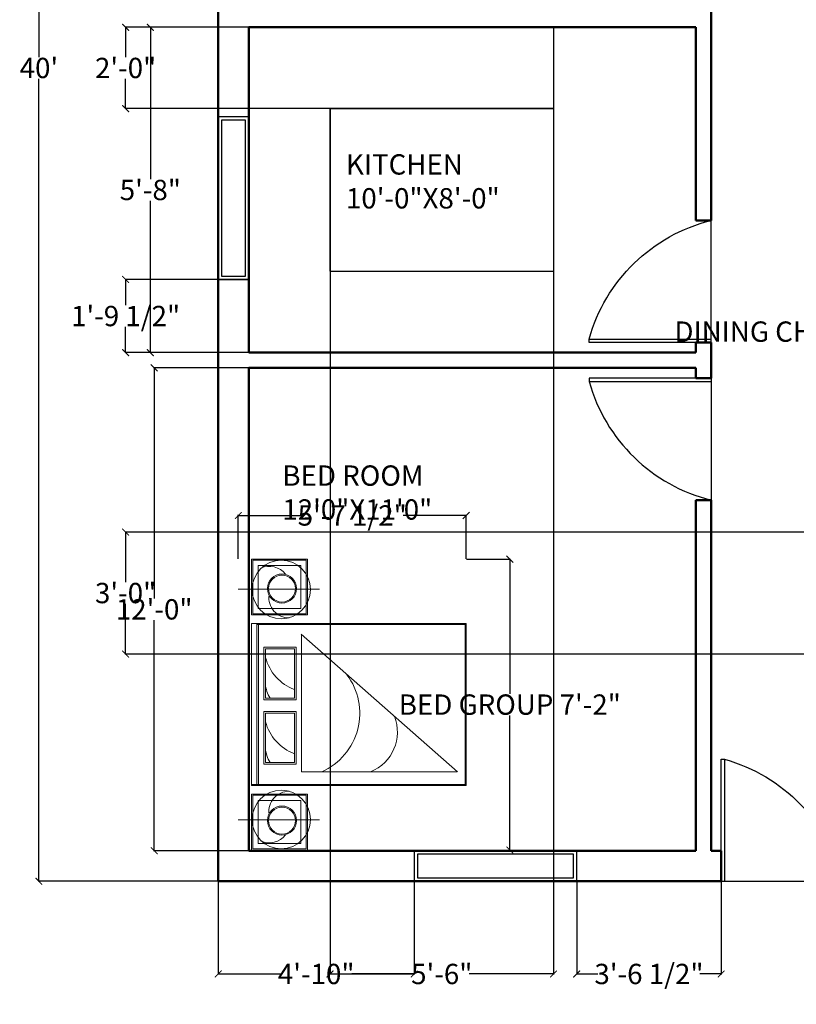
# Model space of a CAD drawing. Units: inches. Extents: x -40 to 418, y 1212 to 1787.
# Tile 1 of 3: x -40 to 189, y 1212 to 1503. Entities that reach past the tile are written whole.
import ezdxf

# ---------------------------------------------------------------- set-up
doc = ezdxf.new("R2010")
doc.units = ezdxf.units.IN
doc.header["$MEASUREMENT"] = 0
for name, color, linetype, lineweight in [('A-ANNO-DIMS', 2, 'Continuous', 18), ('A-AREA-IDEN', 7, 'Continuous', 25), ('A-DOOR', 4, 'Continuous', 25), ('A-FLOR-FIXT', 9, 'Continuous', 25), ('A-FURN', 8, 'Continuous', 18), ('A-GLAZ', 4, 'Continuous', 25), ('A-WALL', 7, 'Continuous', 50)]:
    doc.layers.add(name, color=color, linetype=linetype, lineweight=lineweight)
doc.styles.get("Standard").update_dxf_attribs({"font": 'arial.ttf'})
doc.dimstyles.get("Standard").update_dxf_attribs({"dimtxt": 6, "dimasz": 2, "dimexe": 0.18, "dimexo": 0.0625, "dimgap": 0.09, "dimtad": 0, "dimtih": 1, "dimtoh": 1, "dimdec": 0, "dimzin": 0, "dimdsep": 46, "dimlunit": 4, "dimtxsty": 'Standard', "dimblk": 'ARCHTICK', "dimcen": 0.09, "dimadec": 0, "dimazin": 0, "dimtfac": 1, "dimtdec": 0, "dimtofl": 0, "dimtmove": 0, "dimatfit": 3, "dimldrblk": 'ARCHTICK', "dimfxl": 1, "dimtolj": 1, "dimtzin": 0, "dimarcsym": 0})

# ---------------------------------------------------------------- blocks, each defined once
blk = doc.blocks.new('_ArchTick')
at = {"color": 0, "linetype": 'ByBlock', "const_width": 0.15}
blk.add_lwpolyline([(-0.5, -0.5), (0.5, 0.5)], dxfattribs=at)
blk = doc.blocks.new('*D5')
at = {"layer": 'A-ANNO-DIMS', "color": 0, "lineweight": -2, "transparency": 16777216}
for p, q in [((18.37, 1728.64), (-34.7, 1728.64)), ((-34.52, 1728.64), (-34.52, 1491.79)), ((-34.52, 1248.64), (-34.52, 1485.48)), ((18.37, 1248.64), (-34.7, 1248.64))]:
    blk.add_line(p, q, dxfattribs=at)
at = {"layer": 'Defpoints', "color": 0, "transparency": 16777216}
for p in [(-34.52, 1728.64), (18.43, 1728.64), (18.43, 1248.64)]:
    blk.add_point(p, dxfattribs=at)
at = {"layer": 'A-ANNO-DIMS', "color": 0, "lineweight": -2, "transparency": 16777216, "xscale": 2, "yscale": 2, "zscale": 2}
for p, rotation in [((-34.52, 1728.64), 90), ((-34.52, 1248.64), 270)]:
    blk.add_blockref('_ArchTick', p, dxfattribs=dict(at, rotation=rotation))
at = {"layer": 'A-ANNO-DIMS', "color": 0, "transparency": 16777216, "insert": (-34.52, 1488.64), "char_height": 6, "attachment_point": 5}
blk.add_mtext("\\A1;40'", dxfattribs=at)
blk = doc.blocks.new('*D8')
at = {"layer": 'A-ANNO-DIMS', "color": 0, "lineweight": -2, "transparency": 16777216}
for p, q in [((27.37, 1500.64), (-1.8, 1500.64)), ((-1.62, 1500.64), (-1.62, 1455.79)), ((-1.62, 1404.64), (-1.62, 1449.48)), ((27.37, 1404.64), (-1.8, 1404.64))]:
    blk.add_line(p, q, dxfattribs=at)
at = {"layer": 'Defpoints', "color": 0, "transparency": 16777216}
for p in [(-1.62, 1500.64), (27.43, 1500.64), (27.43, 1404.64)]:
    blk.add_point(p, dxfattribs=at)
at = {"layer": 'A-ANNO-DIMS', "color": 0, "lineweight": -2, "transparency": 16777216, "xscale": 2, "yscale": 2, "zscale": 2}
for p, rotation in [((-1.62, 1500.64), 90), ((-1.62, 1404.64), 270)]:
    blk.add_blockref('_ArchTick', p, dxfattribs=dict(at, rotation=rotation))
at = {"layer": 'A-ANNO-DIMS', "color": 0, "transparency": 16777216, "insert": (-1.62, 1452.64), "char_height": 6, "attachment_point": 5}
blk.add_mtext('\\A1;5\'-8"', dxfattribs=at)
blk = doc.blocks.new('*D9')
at = {"layer": 'A-ANNO-DIMS', "color": 0, "lineweight": -2, "transparency": 16777216}
for p, q in [((27.37, 1400.14), (-0.66, 1400.14)), ((-0.48, 1400.14), (-0.48, 1332.04)), ((-0.48, 1257.64), (-0.48, 1325.73)), ((27.37, 1257.64), (-0.66, 1257.64))]:
    blk.add_line(p, q, dxfattribs=at)
at = {"layer": 'Defpoints', "color": 0, "transparency": 16777216}
for p in [(-0.48, 1400.14), (27.43, 1400.14), (27.43, 1257.64)]:
    blk.add_point(p, dxfattribs=at)
at = {"layer": 'A-ANNO-DIMS', "color": 0, "lineweight": -2, "transparency": 16777216, "xscale": 2, "yscale": 2, "zscale": 2}
for p, rotation in [((-0.48, 1400.14), 90), ((-0.48, 1257.64), 270)]:
    blk.add_blockref('_ArchTick', p, dxfattribs=dict(at, rotation=rotation))
at = {"layer": 'A-ANNO-DIMS', "color": 0, "transparency": 16777216, "insert": (-0.48, 1328.89), "char_height": 6, "attachment_point": 5}
blk.add_mtext('\\A1;12\'-0"', dxfattribs=at)
blk = doc.blocks.new('DESDFGHJUI')
for p, q in [((-198.91, 1688.99), (-198.91, 1729.95)), ((-82.83, 1688.99), (-82.83, 1729.95)), ((-214.04, 1695.16), (-214.04, 1723.24)), ((-214.04, 1723.24), (-185.96, 1723.24)), ((-213.5, 1695.7), (-213.5, 1722.7)), ((-213.5, 1722.7), (-186.5, 1722.7)), ((-210.8, 1698.4), (-210.8, 1720)), ((-210.8, 1720), (-189.2, 1720)), ((-189.2, 1720), (-189.2, 1698.4)), ((-186.5, 1722.7), (-186.5, 1695.7)), ((-185.96, 1723.24), (-185.96, 1695.16)), ((-181.64, 1723.24), (-181.64, 1615.24)), ((-181.64, 1723.24), (-100.1, 1723.24)), ((-181.64, 1720.54), (-100.1, 1720.54)), ((-181.64, 1719.73), (-100.1, 1719.73)), ((-181.1, 1723.24), (-181.1, 1615.24)), ((-100.64, 1720.54), (-100.64, 1615.24)), ((-100.1, 1723.24), (-100.1, 1615.24)), ((-67.7, 1723.24), (-95.78, 1723.24)), ((-95.78, 1723.24), (-95.78, 1695.16)), ((-68.24, 1722.7), (-95.24, 1722.7)), ((-95.24, 1722.7), (-95.24, 1695.7)), ((-70.94, 1720), (-92.54, 1720)), ((-92.54, 1720), (-92.54, 1698.4)), ((-70.94, 1698.4), (-70.94, 1720)), ((-68.24, 1695.7), (-68.24, 1722.7)), ((-67.7, 1695.16), (-67.7, 1723.24)), ((-170.78, 1700.83), (-170.78, 1717.03)), ((-170.78, 1717.03), (-144.32, 1717.03)), ((-169.97, 1701.64), (-169.97, 1716.22)), ((-169.97, 1716.22), (-145.13, 1716.22)), ((-145.13, 1716.22), (-145.13, 1701.64)), ((-144.32, 1717.03), (-144.32, 1700.83)), ((-138.48, 1700.83), (-138.48, 1717.03)), ((-138.48, 1717.03), (-112.02, 1717.03)), ((-137.67, 1701.64), (-137.67, 1716.22)), ((-137.67, 1716.22), (-112.83, 1716.22)), ((-112.83, 1716.22), (-112.83, 1701.64)), ((-112.02, 1717.03), (-112.02, 1700.83)), ((-170.78, 1700.83), (-144.32, 1700.83)), ((-169.97, 1701.64), (-145.13, 1701.64)), ((-138.48, 1700.83), (-112.02, 1700.83)), ((-137.67, 1701.64), (-112.83, 1701.64)), ((-185.96, 1695.16), (-214.04, 1695.16)), ((-186.5, 1695.7), (-213.5, 1695.7)), ((-189.2, 1698.4), (-210.8, 1698.4)), ((-174.68, 1619.61), (-105.47, 1698.21)), ((-174.64, 1619.8), (-174.64, 1698.13)), ((-174.64, 1698.13), (-105.54, 1698.13)), ((-95.78, 1695.16), (-67.7, 1695.16)), ((-95.24, 1695.7), (-68.24, 1695.7)), ((-92.54, 1698.4), (-70.94, 1698.4)), ((-131.52, 1615.74), (-181.64, 1615.74)), ((-100.1, 1615.24), (-181.64, 1615.24)), ((-100.1, 1615.78), (-175.16, 1615.78))]:
    blk.add_line(p, q)
for centre, radius in [((-198.74, 1708.29), 14.73), ((-83.01, 1708.29), 14.73), ((-199.23, 1707.96), 7.32), ((-199.23, 1707.96), 6.78), ((-82.52, 1707.96), 7.32), ((-82.52, 1707.96), 6.78)]:
    blk.add_circle(centre, radius)
for centre, radius, start, end in [((-200.04, 1714.33), 10.36, 155.9567, 231.7564), ((-194.74, 1704.25), 10.3, 0.4104, 96.764), ((-161.57, 1700.2), 16.13, 94.4656, 121.4122), ((-143.54, 1693.44), 23.54, 104.6626, 159.6122), ((-129.26, 1700.2), 16.13, 94.4656, 121.4122), ((-111.24, 1693.44), 23.54, 104.6626, 159.6122), ((-87.01, 1704.25), 10.3, 83.236, 179.5896), ((-81.71, 1714.33), 10.36, 308.2436, 24.0433), ((-145.2, 1701.08), 32.28, 204.0563, 306.8492), ((-154.7, 1671.44), 21.57, 202.1275, 291.5505)]:
    blk.add_arc(centre, radius, start, end)
blk = doc.blocks.new('EREGTHYGUI')
for p, q in [((195.43, 1607.14), (194.43, 1607.14)), ((194.43, 1607.14), (194.43, 1571.14)), ((195.43, 1571.14), (195.43, 1607.14)), ((195.43, 1571.14), (159.43, 1571.14))]:
    blk.add_line(p, q)
blk.add_arc((207.79, 1559.14), 49.82, 105.5486, 166.0653)
blk = doc.blocks.new('WIN-48IN')
for points in [[(0, 0), (9, 0), (9, 48), (0, 48)], [(1, 1), (8, 1), (8, 47), (1, 47)]]:
    blk.add_lwpolyline(points, close=True)
blk = doc.blocks.new('*D21')
at = {"layer": 'A-ANNO-DIMS', "color": 0, "lineweight": -2, "transparency": 16777216}
for p, q in [((253.98, 1414.1), (253.98, 1410.66)), ((276.18, 1414.1), (276.18, 1410.66)), ((253.98, 1410.84), (251.98, 1410.84)), ((276.18, 1410.84), (253.98, 1410.84))]:
    blk.add_line(p, q, dxfattribs=at)
at = {"layer": 'Defpoints', "color": 0, "transparency": 16777216}
for p in [(253.98, 1414.17), (276.18, 1414.17), (253.98, 1410.84)]:
    blk.add_point(p, dxfattribs=at)
at = {"layer": 'A-ANNO-DIMS', "color": 0, "lineweight": -2, "transparency": 16777216, "xscale": 2, "yscale": 2, "zscale": 2}
for p, rotation in [((253.98, 1410.84), 179.9999999999912), ((276.18, 1410.84), 359.9999999999912)]:
    blk.add_blockref('_ArchTick', p, dxfattribs=dict(at, rotation=rotation))
at = {"layer": 'A-ANNO-DIMS', "color": 0, "transparency": 16777216, "insert": (201.38, 1410.84), "char_height": 6, "attachment_point": 5}
blk.add_mtext('\\A1;DINING CHAIR 1\'-10" TYP.', dxfattribs=at)
blk = doc.blocks.new('*D25')
at = {"layer": 'A-ANNO-DIMS', "color": 0, "lineweight": -2, "transparency": 16777216}
for p, q in [((91.7, 1343.71), (104.7, 1343.71)), ((104.52, 1343.71), (104.52, 1303.98)), ((104.52, 1257.86), (104.52, 1297.59)), ((91.7, 1257.86), (104.7, 1257.86))]:
    blk.add_line(p, q, dxfattribs=at)
at = {"layer": 'Defpoints', "color": 0, "transparency": 16777216}
for p in [(91.64, 1343.71), (104.52, 1343.71), (91.64, 1257.86)]:
    blk.add_point(p, dxfattribs=at)
at = {"layer": 'A-ANNO-DIMS', "color": 0, "lineweight": -2, "transparency": 16777216, "xscale": 2, "yscale": 2, "zscale": 2}
for p, rotation in [((104.52, 1343.71), 90), ((104.52, 1257.86), 270)]:
    blk.add_blockref('_ArchTick', p, dxfattribs=dict(at, rotation=rotation))
at = {"layer": 'A-ANNO-DIMS', "color": 0, "transparency": 16777216, "insert": (104.52, 1300.78), "char_height": 6, "attachment_point": 5}
blk.add_mtext('\\A1;BED GROUP 7\'-2"', dxfattribs=at)
blk = doc.blocks.new('*D26')
at = {"layer": 'A-ANNO-DIMS', "color": 0, "lineweight": -2, "transparency": 16777216}
for p, q in [((24.35, 1343.77), (24.35, 1356.77)), ((24.35, 1356.59), (42.94, 1356.59)), ((91.64, 1356.59), (73.05, 1356.59)), ((91.64, 1343.77), (91.64, 1356.77))]:
    blk.add_line(p, q, dxfattribs=at)
at = {"layer": 'Defpoints', "color": 0, "transparency": 16777216}
for p in [(24.35, 1356.59), (24.35, 1343.71), (91.64, 1343.71)]:
    blk.add_point(p, dxfattribs=at)
at = {"layer": 'A-ANNO-DIMS', "color": 0, "lineweight": -2, "transparency": 16777216, "xscale": 2, "yscale": 2, "zscale": 2, "rotation": 180}
blk.add_blockref('_ArchTick', (24.35, 1356.59), dxfattribs=at)
at = {"layer": 'A-ANNO-DIMS', "color": 0, "lineweight": -2, "transparency": 16777216, "xscale": 2, "yscale": 2, "zscale": 2}
blk.add_blockref('_ArchTick', (91.64, 1356.59), dxfattribs=at)
at = {"layer": 'A-ANNO-DIMS', "color": 0, "transparency": 16777216, "insert": (57.99, 1356.59), "char_height": 6, "attachment_point": 5}
blk.add_mtext('\\A1;5\'-7 1/2"', dxfattribs=at)
blk = doc.blocks.new('*D33')
at = {"layer": 'A-ANNO-DIMS', "color": 0, "lineweight": -2, "transparency": 16777216}
for p, q in [((18.43, 1248.57), (18.43, 1221.11)), ((76.28, 1248.57), (76.28, 1221.11)), ((18.43, 1221.29), (36.84, 1221.29)), ((76.28, 1221.29), (57.87, 1221.29))]:
    blk.add_line(p, q, dxfattribs=at)
at = {"layer": 'Defpoints', "color": 0, "transparency": 16777216}
for p in [(18.43, 1248.64), (76.28, 1248.64), (76.28, 1221.29)]:
    blk.add_point(p, dxfattribs=at)
at = {"layer": 'A-ANNO-DIMS', "color": 0, "lineweight": -2, "transparency": 16777216, "xscale": 2, "yscale": 2, "zscale": 2, "rotation": 180}
blk.add_blockref('_ArchTick', (18.43, 1221.29), dxfattribs=at)
at = {"layer": 'A-ANNO-DIMS', "color": 0, "lineweight": -2, "transparency": 16777216, "xscale": 2, "yscale": 2, "zscale": 2}
blk.add_blockref('_ArchTick', (76.28, 1221.29), dxfattribs=at)
at = {"layer": 'A-ANNO-DIMS', "color": 0, "transparency": 16777216, "insert": (47.36, 1221.29), "char_height": 6, "attachment_point": 5}
blk.add_mtext('\\A1;4\'-10"', dxfattribs=at)
blk = doc.blocks.new('*D34')
at = {"layer": 'A-ANNO-DIMS', "color": 0, "lineweight": -2, "transparency": 16777216}
for p, q in [((124.28, 1248.57), (124.28, 1221.11)), ((166.93, 1248.57), (166.93, 1221.11)), ((124.28, 1221.29), (130.55, 1221.29)), ((166.93, 1221.29), (160.66, 1221.29))]:
    blk.add_line(p, q, dxfattribs=at)
at = {"layer": 'Defpoints', "color": 0, "transparency": 16777216}
for p in [(124.28, 1248.64), (166.93, 1248.64), (166.93, 1221.29)]:
    blk.add_point(p, dxfattribs=at)
at = {"layer": 'A-ANNO-DIMS', "color": 0, "lineweight": -2, "transparency": 16777216, "xscale": 2, "yscale": 2, "zscale": 2, "rotation": 180}
blk.add_blockref('_ArchTick', (124.28, 1221.29), dxfattribs=at)
at = {"layer": 'A-ANNO-DIMS', "color": 0, "lineweight": -2, "transparency": 16777216, "xscale": 2, "yscale": 2, "zscale": 2}
blk.add_blockref('_ArchTick', (166.93, 1221.29), dxfattribs=at)
at = {"layer": 'A-ANNO-DIMS', "color": 0, "transparency": 16777216, "insert": (145.61, 1221.29), "char_height": 6, "attachment_point": 5}
blk.add_mtext('\\A1;3\'-6 1/2"', dxfattribs=at)
blk = doc.blocks.new('*D38')
at = {"layer": 'A-ANNO-DIMS', "color": 0, "lineweight": -2, "transparency": 16777216}
for p, q in [((27.37, 1426.24), (-9.1, 1426.24)), ((-8.92, 1426.24), (-8.92, 1418.63)), ((-8.92, 1404.64), (-8.92, 1412.25)), ((27.37, 1404.64), (-9.1, 1404.64))]:
    blk.add_line(p, q, dxfattribs=at)
at = {"layer": 'Defpoints', "color": 0, "transparency": 16777216}
for p in [(-8.92, 1426.24), (27.43, 1426.24), (27.43, 1404.64)]:
    blk.add_point(p, dxfattribs=at)
at = {"layer": 'A-ANNO-DIMS', "color": 0, "lineweight": -2, "transparency": 16777216, "xscale": 2, "yscale": 2, "zscale": 2}
for p, rotation in [((-8.92, 1426.24), 90), ((-8.92, 1404.64), 270)]:
    blk.add_blockref('_ArchTick', p, dxfattribs=dict(at, rotation=rotation))
at = {"layer": 'A-ANNO-DIMS', "color": 0, "transparency": 16777216, "insert": (-8.92, 1415.44), "char_height": 6, "attachment_point": 5}
blk.add_mtext('\\A1;1\'-9 1/2"', dxfattribs=at)
blk = doc.blocks.new('*D41')
at = {"layer": 'A-ANNO-DIMS', "color": 0, "lineweight": -2, "transparency": 16777216}
for p, q in [((284.69, 1351.7), (-9.1, 1351.7)), ((-8.92, 1351.7), (-8.92, 1336.86)), ((-8.92, 1315.7), (-8.92, 1330.55)), ((284.69, 1315.7), (-9.1, 1315.7))]:
    blk.add_line(p, q, dxfattribs=at)
at = {"layer": 'Defpoints', "color": 0, "transparency": 16777216}
for p in [(-8.92, 1351.7), (284.75, 1351.7), (284.75, 1315.7)]:
    blk.add_point(p, dxfattribs=at)
at = {"layer": 'A-ANNO-DIMS', "color": 0, "lineweight": -2, "transparency": 16777216, "xscale": 2, "yscale": 2, "zscale": 2}
for p, rotation in [((-8.92, 1351.7), 90), ((-8.92, 1315.7), 270)]:
    blk.add_blockref('_ArchTick', p, dxfattribs=dict(at, rotation=rotation))
at = {"layer": 'A-ANNO-DIMS', "color": 0, "transparency": 16777216, "insert": (-8.92, 1333.7), "char_height": 6, "attachment_point": 5}
blk.add_mtext('\\A1;3\'-0"', dxfattribs=at)
blk = doc.blocks.new('*D45')
at = {"layer": 'A-ANNO-DIMS', "color": 0, "lineweight": -2, "transparency": 16777216}
for p, q in [((117.37, 1500.64), (-9.1, 1500.64)), ((-8.92, 1500.64), (-8.92, 1491.79)), ((-8.92, 1476.64), (-8.92, 1485.48)), ((117.37, 1476.64), (-9.1, 1476.64))]:
    blk.add_line(p, q, dxfattribs=at)
at = {"layer": 'Defpoints', "color": 0, "transparency": 16777216}
for p in [(-8.92, 1500.64), (117.43, 1500.64), (117.43, 1476.64)]:
    blk.add_point(p, dxfattribs=at)
at = {"layer": 'A-ANNO-DIMS', "color": 0, "lineweight": -2, "transparency": 16777216, "xscale": 2, "yscale": 2, "zscale": 2}
for p, rotation in [((-8.92, 1500.64), 90), ((-8.92, 1476.64), 270)]:
    blk.add_blockref('_ArchTick', p, dxfattribs=dict(at, rotation=rotation))
at = {"layer": 'A-ANNO-DIMS', "color": 0, "transparency": 16777216, "insert": (-8.92, 1488.64), "char_height": 6, "attachment_point": 5}
blk.add_mtext('\\A1;2\'-0"', dxfattribs=at)
blk = doc.blocks.new('*D46')
at = {"layer": 'A-ANNO-DIMS', "color": 0, "lineweight": -2, "transparency": 16777216}
for p, q in [((51.43, 1476.57), (51.43, 1221.11)), ((117.43, 1476.57), (117.43, 1221.11)), ((51.43, 1221.29), (76.37, 1221.29)), ((117.43, 1221.29), (92.5, 1221.29))]:
    blk.add_line(p, q, dxfattribs=at)
at = {"layer": 'Defpoints', "color": 0, "transparency": 16777216}
for p in [(51.43, 1476.64), (117.43, 1476.64), (117.43, 1221.29)]:
    blk.add_point(p, dxfattribs=at)
at = {"layer": 'A-ANNO-DIMS', "color": 0, "lineweight": -2, "transparency": 16777216, "xscale": 2, "yscale": 2, "zscale": 2, "rotation": 180}
blk.add_blockref('_ArchTick', (51.43, 1221.29), dxfattribs=at)
at = {"layer": 'A-ANNO-DIMS', "color": 0, "lineweight": -2, "transparency": 16777216, "xscale": 2, "yscale": 2, "zscale": 2}
blk.add_blockref('_ArchTick', (117.43, 1221.29), dxfattribs=at)
at = {"layer": 'A-ANNO-DIMS', "color": 0, "transparency": 16777216, "insert": (84.43, 1221.29), "char_height": 6, "attachment_point": 5}
blk.add_mtext('\\A1;5\'-6"', dxfattribs=at)

msp = doc.modelspace()

# ---------------------------------------------------------------- linework, layer by layer
at = {"layer": 'A-FLOR-FIXT'}
for p, q in [((117.43, 1500.64), (117.43, 1476.64)), ((51.43, 1476.64), (117.43, 1476.64)), ((51.43, 1428.64), (51.43, 1476.64)), ((51.43, 1428.64), (117.43, 1428.64)), ((117.43, 1428.64), (117.43, 1404.64))]:
    msp.add_line(p, q, dxfattribs=at)
at = {"layer": 'A-WALL'}
for p, q in [((18.43, 1248.64), (18.43, 1728.64)), ((163.93, 1443.64), (163.93, 1505.14)), ((27.43, 1404.64), (27.43, 1500.64)), ((27.43, 1500.64), (159.43, 1500.64)), ((159.43, 1443.64), (159.43, 1500.64)), ((159.43, 1443.64), (163.93, 1443.64)), ((159.43, 1404.64), (159.43, 1407.64)), ((159.43, 1407.64), (163.93, 1407.64)), ((163.93, 1404.64), (163.93, 1407.64)), ((27.43, 1404.64), (159.43, 1404.64)), ((163.93, 1397.14), (163.93, 1404.64)), ((27.43, 1257.64), (27.43, 1400.14)), ((27.43, 1400.14), (159.43, 1400.14)), ((159.43, 1397.14), (159.43, 1400.14)), ((159.43, 1397.14), (163.93, 1397.14)), ((159.43, 1257.64), (159.43, 1361.14)), ((159.43, 1361.14), (163.93, 1361.14)), ((163.93, 1257.64), (163.93, 1361.14)), ((159.43, 1257.64), (27.43, 1257.64)), ((166.93, 1257.64), (163.93, 1257.64)), ((166.93, 1248.64), (166.93, 1257.64)), ((166.93, 1248.64), (18.43, 1248.64))]:
    msp.add_line(p, q, dxfattribs=at)

# ---------------------------------------------------------------- block references
at = {"layer": 'A-DOOR', "xscale": -1, "rotation": 90}
msp.add_blockref('EREGTHYGUI', (1735.07, 1603.07), dxfattribs=at)
at = {"layer": 'A-DOOR', "rotation": 90}
msp.add_blockref('EREGTHYGUI', (1735.07, 1201.7), dxfattribs=at)
at = {"layer": 'A-DOOR', "xscale": -1}
msp.add_blockref('EREGTHYGUI', (362.37, -322.5), dxfattribs=at)
at = {"layer": 'A-FURN', "xscale": 0.5866395626792551, "yscale": 0.5866395626792551, "zscale": 0.5866395626792551, "rotation": 90}
msp.add_blockref('DESDFGHJUI', (1039.2, 1383.43), dxfattribs=at)
at = {"layer": 'A-GLAZ'}
msp.add_blockref('WIN-48IN', (18.43, 1426.24), dxfattribs=at)
at = {"layer": 'A-GLAZ', "rotation": 269.9999999999991}
msp.add_blockref('WIN-48IN', (76.28, 1257.64), dxfattribs=at)

# ---------------------------------------------------------------- texts
at = {"layer": 'A-AREA-IDEN', "char_height": 6, "attachment_point": 1}
for s, width, insert in [('KITCHEN\\P10\'-0"X8\'-0"', 281.2427, (56.14, 1463.18)), ('BED ROOM\\P12\'0"X11\'0"', 72.7243, (37.36, 1371.36))]:
    msp.add_mtext_dynamic_manual_height_columns(s, width=width, gutter_width=30, heights=[0], dxfattribs=dict(at, insert=insert))

# ---------------------------------------------------------------- dimensions: what is measured, and where the dimension line sits
at = {"layer": 'A-ANNO-DIMS'}
for base, p1, p2, angle, override, picture, middle in [((-34.52, 1728.64), (18.43, 1248.64), (18.43, 1728.64), 90, {"dimclrd": 0, "dimclre": 0, "dimclrt": 0}, '*D5', (-34.52, 1488.64)), ((-8.92, 1500.64), (117.43, 1476.64), (117.43, 1500.64), 90, {"dimdec": 1, "dimlfac": 1, "dimrnd": 0, "dimzin": 1, "dimdsep": 46, "dimlunit": 4, "dimfrac": 2}, '*D45', (-8.92, 1488.64)), ((-8.92, 1426.24), (27.43, 1404.64), (27.43, 1426.24), 90, {"dimdec": 1, "dimlfac": 1, "dimrnd": 0, "dimzin": 1, "dimdsep": 46, "dimlunit": 4, "dimfrac": 2}, '*D38', (-8.92, 1415.44)), ((24.35, 1356.59), (91.64, 1343.71), (24.35, 1343.71), 180, {"dimdec": 1, "dimlfac": 1, "dimrnd": 0, "dimzin": 1, "dimdsep": 46, "dimlunit": 4, "dimfrac": 2}, '*D26', (57.99, 1356.59)), ((-8.92, 1351.7), (284.75, 1315.7), (284.75, 1351.7), 90, {"dimdec": 1, "dimlfac": 1, "dimrnd": 0, "dimzin": 1, "dimdsep": 46, "dimlunit": 4, "dimfrac": 2}, '*D41', (-8.92, 1333.7))]:
    dim = msp.add_linear_dim(base=base, p1=p1, p2=p2, angle=angle, dimstyle='Standard', override=override, dxfattribs=at)
    dim.commit()
    dim.dimension.update_dxf_attribs({"geometry": picture, "text_midpoint": middle})
for base, p1, p2, angle, text, override, picture, middle in [((-1.62, 1500.64), (27.43, 1404.64), (27.43, 1500.64), 90, '5\'-8"', {"dimclrd": 0, "dimclre": 0, "dimclrt": 0}, '*D8', (-1.62, 1452.64)), ((253.98, 1410.84), (276.18, 1414.17), (253.98, 1414.17), 180, 'DINING CHAIR <> TYP.', {"dimdec": 1, "dimlfac": 1, "dimrnd": 0, "dimzin": 1, "dimdsep": 46, "dimlunit": 4, "dimfrac": 2}, '*D21', (201.38, 1410.84)), ((-0.48, 1400.14), (27.43, 1257.64), (27.43, 1400.14), 90, '12\'-0"', {"dimclrd": 0, "dimclre": 0, "dimclrt": 0}, '*D9', (-0.48, 1328.89)), ((104.5194, 1343.7093), (91.642, 1257.8604), (91.642, 1343.7093), 90, 'BED GROUP <>', {"dimdec": 1, "dimlfac": 1, "dimrnd": 0, "dimzin": 1, "dimdsep": 46, "dimlunit": 4, "dimfrac": 2}, '*D25', (104.5194, 1300.7849))]:
    dim = msp.add_linear_dim(base=base, p1=p1, p2=p2, angle=angle, text=text, dimstyle='Standard', override=override, dxfattribs=at)
    dim.commit()
    dim.dimension.update_dxf_attribs({"geometry": picture, "text_midpoint": middle})
for base, p1, p2, picture, middle in [((117.43, 1221.29), (51.43, 1476.64), (117.43, 1476.64), '*D46', (84.43, 1221.29)), ((76.2794, 1221.2872), (18.4349, 1248.6372), (76.2794, 1248.6372), '*D33', (47.3571, 1221.2872)), ((166.9349, 1221.2872), (124.2794, 1248.6372), (166.9349, 1248.6372), '*D34', (145.6071, 1221.2872))]:
    dim = msp.add_linear_dim(base=base, p1=p1, p2=p2, dimstyle='Standard', override={"dimdec": 1, "dimlfac": 1, "dimrnd": 0, "dimzin": 1, "dimdsep": 46, "dimlunit": 4, "dimfrac": 2}, dxfattribs=at)
    dim.commit()
    dim.dimension.update_dxf_attribs({"geometry": picture, "text_midpoint": middle})

doc.saveas('drawing.dxf')
